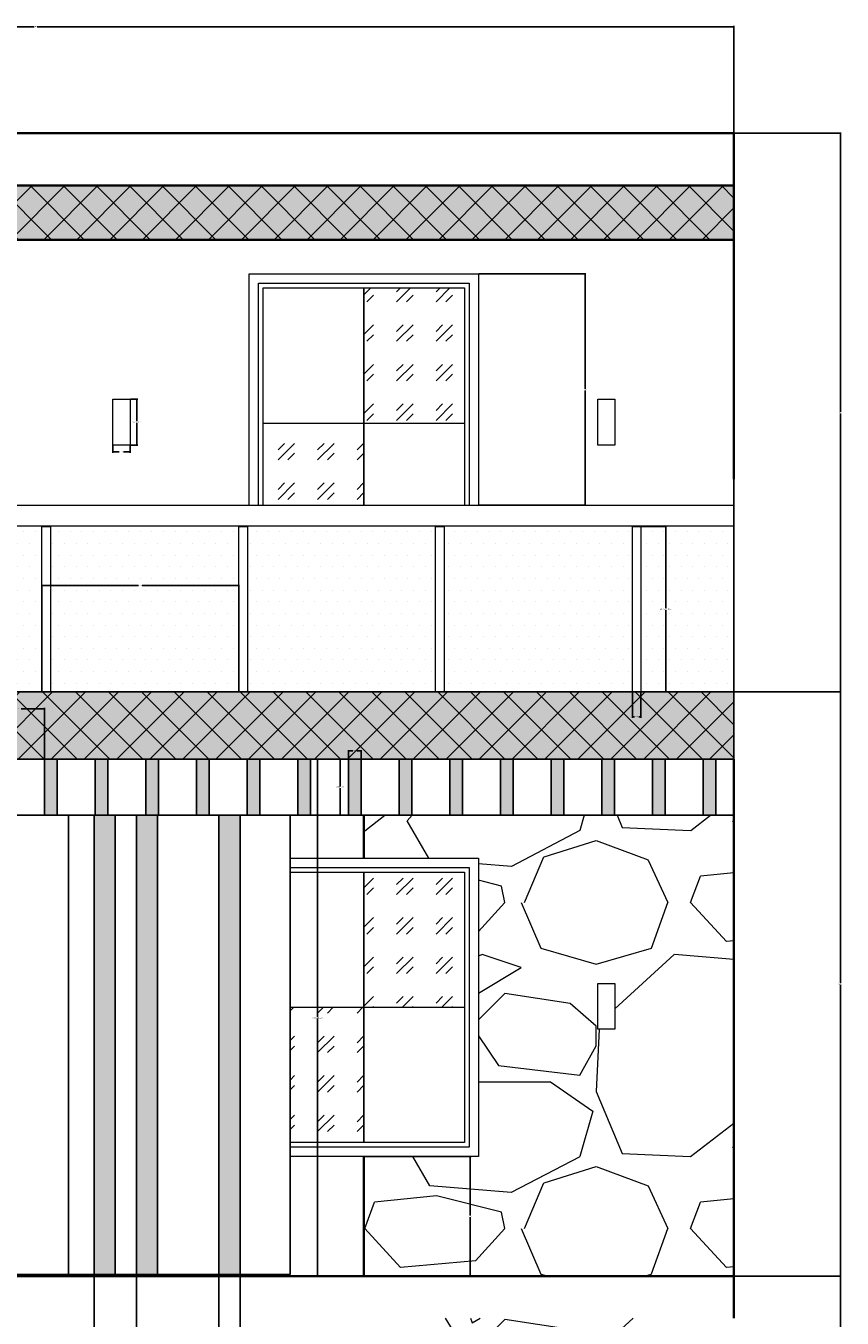
# Model space of a CAD drawing. Units: inches. Extents: x -13 to 333, y -76 to 399.
# Tile 3 of 3: x 158 to 333, y 121 to 399. Entities that reach past the tile are written whole.
import ezdxf

# ---------------------------------------------------------------- set-up
doc = ezdxf.new("R2010")
doc.units = ezdxf.units.IN
doc.header["$MEASUREMENT"] = 0
for name, color, linetype, lineweight in [('A-ANNO-DIMS', 2, 'Continuous', 18), ('A-ELEV-TRIM', 7, 'Continuous', 25), ('A-FLOR', 7, 'Continuous', 35), ('A-FLOR-HRAL', 4, 'Continuous', 20), ('A-FLOR-HRAL-PATT', 8, 'Continuous', 13), ('A-GLAZ', 4, 'Continuous', 18), ('A-GLAZ-PATT', 8, 'Continuous', 13), ('A-ROOF', 7, 'Continuous', 35), ('A-WALL', 7, 'Continuous', 35), ('A-WALL-PATT', 252, 'Continuous', 13), ('E-LITE-EXTR', 2, 'Continuous', 18)]:
    doc.layers.add(name, color=color, linetype=linetype, lineweight=lineweight)
doc.styles.get("Standard").update_dxf_attribs({"font": 'arial.ttf'})
doc.dimstyles.get("Standard").update_dxf_attribs({"dimtxt": 0.18, "dimasz": 0.18, "dimexe": 0.18, "dimexo": 0.0625, "dimgap": 0.09, "dimtad": 0, "dimtih": 1, "dimtoh": 1, "dimdec": 4, "dimzin": 0, "dimdsep": 46, "dimtxsty": 'Standard', "dimcen": 0.09, "dimadec": 0, "dimazin": 0, "dimtfac": 1, "dimtdec": 4, "dimtofl": 0, "dimtmove": 0, "dimatfit": 3, "dimfxl": 1, "dimtolj": 1, "dimtzin": 0, "dimarcsym": 0})

# ---------------------------------------------------------------- blocks, each defined once
blk = doc.blocks.new('LIGHT-WALL-SCONCE')
blk.add_lwpolyline([(0, 9.86), (3.7, 9.86), (3.7, 0), (0, 0)], close=True)
blk = doc.blocks.new('FASCIA-BATTEN')
blk.add_lwpolyline([(0, 12), (0, 0), (2.72, 0), (2.72, 12)])
blk = doc.blocks.new('GUARD-POST-TERRACE')
blk.add_lwpolyline([(0, 35.57), (1.84, 35.57), (1.84, 0), (0, 0)], close=True)
blk = doc.blocks.new('FACADE-VERTICAL-STRIP')
for points in [[(4.54, 111), (0, 111)], [(0, 99), (0, 0), (4.54, 0), (4.54, 99)]]:
    blk.add_lwpolyline(points)
blk = doc.blocks.new('*D6')
at = {"layer": 'A-ANNO-DIMS', "color": 0, "lineweight": -2, "transparency": 16777216}
for p, q in [((227.2, 241.18), (225.28, 241.18)), ((225.46, 241), (225.46, 235.36)), ((225.46, 229.36), (225.46, 235)), ((227.2, 229.18), (225.28, 229.18))]:
    blk.add_line(p, q, dxfattribs=at)
at = {"layer": 'A-ANNO-DIMS', "color": 0, "transparency": 16777216}
for points in [[(225.43, 241), (225.49, 241), (225.46, 241.18)], [(225.43, 229.36), (225.49, 229.36), (225.46, 229.18)]]:
    blk.add_solid(points, dxfattribs=at)
at = {"layer": 'Defpoints', "color": 0, "transparency": 16777216}
for p in [(225.46, 241.18), (227.26, 241.18), (227.26, 229.18)]:
    blk.add_point(p, dxfattribs=at)
at = {"layer": 'A-ANNO-DIMS', "color": 0, "transparency": 16777216, "insert": (225.46, 235.18), "char_height": 0.18, "attachment_point": 5}
blk.add_mtext('\\A1;BATTEN 12 TYP.', dxfattribs=at)
blk = doc.blocks.new('*D7')
at = {"layer": 'A-ANNO-DIMS', "color": 0, "lineweight": -2, "transparency": 16777216}
for p, q in [((227.26, 241.24), (227.26, 243.16)), ((227.44, 242.98), (228.17, 242.98)), ((229.8, 242.98), (229.08, 242.98)), ((229.98, 241.24), (229.98, 243.16))]:
    blk.add_line(p, q, dxfattribs=at)
at = {"layer": 'A-ANNO-DIMS', "color": 0, "transparency": 16777216}
for points in [[(227.44, 243.01), (227.44, 242.95), (227.26, 242.98)], [(229.8, 243.01), (229.8, 242.95), (229.98, 242.98)]]:
    blk.add_solid(points, dxfattribs=at)
at = {"layer": 'Defpoints', "color": 0, "transparency": 16777216}
for p in [(229.98, 242.98), (227.26, 241.18), (229.98, 241.18)]:
    blk.add_point(p, dxfattribs=at)
at = {"layer": 'A-ANNO-DIMS', "color": 0, "transparency": 16777216, "insert": (228.62, 242.98), "char_height": 0.18, "attachment_point": 5}
blk.add_mtext('\\A1;3 TYP.', dxfattribs=at)
blk = doc.blocks.new('*D8')
at = {"layer": 'A-ANNO-DIMS', "color": 0, "lineweight": -2, "transparency": 16777216}
for p, q in [((180.41, 318.52), (182.01, 318.52)), ((181.83, 318.34), (181.83, 313.77)), ((181.83, 308.83), (181.83, 313.4)), ((180.41, 308.65), (182.01, 308.65))]:
    blk.add_line(p, q, dxfattribs=at)
at = {"layer": 'A-ANNO-DIMS', "color": 0, "transparency": 16777216}
for points in [[(181.8, 318.34), (181.86, 318.34), (181.83, 318.52)], [(181.8, 308.83), (181.86, 308.83), (181.83, 308.65)]]:
    blk.add_solid(points, dxfattribs=at)
at = {"layer": 'Defpoints', "color": 0, "transparency": 16777216}
for p in [(180.35, 318.52), (181.83, 318.52), (180.35, 308.65)]:
    blk.add_point(p, dxfattribs=at)
at = {"layer": 'A-ANNO-DIMS', "color": 0, "transparency": 16777216, "insert": (181.83, 313.59), "char_height": 0.18, "attachment_point": 5}
blk.add_mtext('\\A1;SCONCE 10 TYP.', dxfattribs=at)
blk = doc.blocks.new('*D9')
at = {"layer": 'A-ANNO-DIMS', "color": 0, "lineweight": -2, "transparency": 16777216}
for p, q in [((176.65, 308.59), (176.65, 307)), ((180.35, 308.59), (180.35, 307)), ((176.83, 307.18), (178.04, 307.18)), ((180.17, 307.18), (178.96, 307.18))]:
    blk.add_line(p, q, dxfattribs=at)
at = {"layer": 'A-ANNO-DIMS', "color": 0, "transparency": 16777216}
for points in [[(176.83, 307.21), (176.83, 307.15), (176.65, 307.18)], [(180.17, 307.21), (180.17, 307.15), (180.35, 307.18)]]:
    blk.add_solid(points, dxfattribs=at)
at = {"layer": 'Defpoints', "color": 0, "transparency": 16777216}
for p in [(176.65, 308.65), (180.35, 308.65), (180.35, 307.18)]:
    blk.add_point(p, dxfattribs=at)
at = {"layer": 'A-ANNO-DIMS', "color": 0, "transparency": 16777216, "insert": (178.5, 307.18), "char_height": 0.18, "attachment_point": 5}
blk.add_mtext('\\A1;4 TYP.', dxfattribs=at)
blk = doc.blocks.new('*D10')
at = {"layer": 'A-ANNO-DIMS', "color": 0, "lineweight": -2, "transparency": 16777216}
for p, q in [((290.15, 291.2), (295.6, 291.2)), ((295.42, 291.02), (295.42, 273.6)), ((295.42, 255.81), (295.42, 273.23)), ((290.15, 255.63), (295.6, 255.63))]:
    blk.add_line(p, q, dxfattribs=at)
at = {"layer": 'A-ANNO-DIMS', "color": 0, "transparency": 16777216}
for points in [[(295.39, 291.02), (295.45, 291.02), (295.42, 291.2)], [(295.39, 255.81), (295.45, 255.81), (295.42, 255.63)]]:
    blk.add_solid(points, dxfattribs=at)
at = {"layer": 'Defpoints', "color": 0, "transparency": 16777216}
for p in [(290.08, 291.2), (295.42, 291.2), (290.08, 255.63)]:
    blk.add_point(p, dxfattribs=at)
at = {"layer": 'A-ANNO-DIMS', "color": 0, "transparency": 16777216, "insert": (295.42, 273.42), "char_height": 0.18, "attachment_point": 5}
blk.add_mtext('\\A1;TERRACE POST 36 TYP.', dxfattribs=at)
blk = doc.blocks.new('*D11')
at = {"layer": 'A-ANNO-DIMS', "color": 0, "lineweight": -2, "transparency": 16777216}
for p, q in [((288.25, 255.57), (288.25, 250.11)), ((290.08, 255.57), (290.08, 250.11)), ((288.43, 250.29), (288.71, 250.29)), ((289.9, 250.29), (289.63, 250.29))]:
    blk.add_line(p, q, dxfattribs=at)
at = {"layer": 'A-ANNO-DIMS', "color": 0, "transparency": 16777216}
for points in [[(288.43, 250.32), (288.43, 250.26), (288.25, 250.29)], [(289.9, 250.32), (289.9, 250.26), (290.08, 250.29)]]:
    blk.add_solid(points, dxfattribs=at)
at = {"layer": 'Defpoints', "color": 0, "transparency": 16777216}
for p in [(288.25, 255.63), (290.08, 255.63), (290.08, 250.29)]:
    blk.add_point(p, dxfattribs=at)
at = {"layer": 'A-ANNO-DIMS', "color": 0, "transparency": 16777216, "insert": (289.17, 250.29), "char_height": 0.18, "attachment_point": 5}
blk.add_mtext('\\A1;2 TYP.', dxfattribs=at)
blk = doc.blocks.new('*D14')
at = {"layer": 'A-ANNO-DIMS', "color": 0, "lineweight": -2, "transparency": 16777216}
for p, q in [((204.05, 241.18), (220.82, 241.18)), ((220.64, 241), (220.64, 185.86)), ((220.64, 130.36), (220.64, 185.49)), ((204.05, 130.18), (220.82, 130.18))]:
    blk.add_line(p, q, dxfattribs=at)
at = {"layer": 'A-ANNO-DIMS', "color": 0, "transparency": 16777216}
for points in [[(220.61, 241), (220.67, 241), (220.64, 241.18)], [(220.61, 130.36), (220.67, 130.36), (220.64, 130.18)]]:
    blk.add_solid(points, dxfattribs=at)
at = {"layer": 'Defpoints', "color": 0, "transparency": 16777216}
for p in [(203.99, 241.18), (220.64, 241.18), (203.99, 130.18)]:
    blk.add_point(p, dxfattribs=at)
at = {"layer": 'A-ANNO-DIMS', "color": 0, "transparency": 16777216, "insert": (220.64, 185.68), "char_height": 0.18, "attachment_point": 5}
blk.add_mtext('\\A1;FACADE STRIP 111 TYP.', dxfattribs=at)
blk = doc.blocks.new('*D15')
at = {"layer": 'A-ANNO-DIMS', "color": 0, "lineweight": -2, "transparency": 16777216}
for p, q in [((199.44, 130.11), (199.44, 113.35)), ((203.99, 130.11), (203.99, 113.35)), ((199.62, 113.53), (201.26, 113.53)), ((203.81, 113.53), (202.17, 113.53))]:
    blk.add_line(p, q, dxfattribs=at)
at = {"layer": 'A-ANNO-DIMS', "color": 0, "transparency": 16777216}
for points in [[(199.62, 113.56), (199.62, 113.5), (199.44, 113.53)], [(203.81, 113.56), (203.81, 113.5), (203.99, 113.53)]]:
    blk.add_solid(points, dxfattribs=at)
at = {"layer": 'Defpoints', "color": 0, "transparency": 16777216}
for p in [(199.44, 130.18), (203.99, 130.18), (203.99, 113.53)]:
    blk.add_point(p, dxfattribs=at)
at = {"layer": 'A-ANNO-DIMS', "color": 0, "transparency": 16777216, "insert": (201.71, 113.53), "char_height": 0.18, "attachment_point": 5}
blk.add_mtext('\\A1;5 TYP.', dxfattribs=at)
blk = doc.blocks.new('*D16')
at = {"layer": 'A-ANNO-DIMS', "color": 0, "lineweight": -2, "transparency": 16777216}
for p, q in [((10.07, 301.43), (10.07, 398.67)), ((10.25, 398.49), (159.78, 398.49)), ((309.89, 398.49), (160.36, 398.49)), ((310.07, 375.69), (310.07, 398.67))]:
    blk.add_line(p, q, dxfattribs=at)
at = {"layer": 'A-ANNO-DIMS', "color": 0, "transparency": 16777216}
for points in [[(10.25, 398.52), (10.25, 398.46), (10.07, 398.49)], [(309.89, 398.52), (309.89, 398.46), (310.07, 398.49)]]:
    blk.add_solid(points, dxfattribs=at)
at = {"layer": 'Defpoints', "color": 0, "transparency": 16777216}
for p in [(310.07, 398.49), (310.07, 375.63), (10.07, 301.36)]:
    blk.add_point(p, dxfattribs=at)
at = {"layer": 'A-ANNO-DIMS', "color": 0, "transparency": 16777216, "insert": (160.07, 398.49), "char_height": 0.18, "attachment_point": 5}
blk.add_mtext('\\A1;300', dxfattribs=at)
blk = doc.blocks.new('*D19')
at = {"layer": 'A-ANNO-DIMS', "color": 0, "lineweight": -2, "transparency": 16777216}
for p, q in [((310.13, 130.18), (333.11, 130.18)), ((332.93, 130), (332.93, 65.86)), ((332.93, 1.36), (332.93, 65.49)), ((310.13, 1.18), (333.11, 1.18))]:
    blk.add_line(p, q, dxfattribs=at)
at = {"layer": 'A-ANNO-DIMS', "color": 0, "transparency": 16777216}
for points in [[(332.9, 130), (332.96, 130), (332.93, 130.18)], [(332.9, 1.36), (332.96, 1.36), (332.93, 1.18)]]:
    blk.add_solid(points, dxfattribs=at)
at = {"layer": 'Defpoints', "color": 0, "transparency": 16777216}
for p in [(310.07, 130.18), (332.93, 130.18), (310.07, 1.18)]:
    blk.add_point(p, dxfattribs=at)
at = {"layer": 'A-ANNO-DIMS', "color": 0, "transparency": 16777216, "insert": (332.93, 65.68), "char_height": 0.18, "attachment_point": 5}
blk.add_mtext('\\A1;129', dxfattribs=at)
blk = doc.blocks.new('*D20')
at = {"layer": 'A-ANNO-DIMS', "color": 0, "lineweight": -2, "transparency": 16777216}
for p, q in [((310.13, 255.63), (333.11, 255.63)), ((332.93, 255.45), (332.93, 193.09)), ((332.93, 130.36), (332.93, 192.72)), ((310.13, 130.18), (333.11, 130.18))]:
    blk.add_line(p, q, dxfattribs=at)
at = {"layer": 'A-ANNO-DIMS', "color": 0, "transparency": 16777216}
for points in [[(332.9, 255.45), (332.96, 255.45), (332.93, 255.63)], [(332.9, 130.36), (332.96, 130.36), (332.93, 130.18)]]:
    blk.add_solid(points, dxfattribs=at)
at = {"layer": 'Defpoints', "color": 0, "transparency": 16777216}
for p in [(310.07, 255.63), (332.93, 255.63), (310.07, 130.18)]:
    blk.add_point(p, dxfattribs=at)
at = {"layer": 'A-ANNO-DIMS', "color": 0, "transparency": 16777216, "insert": (332.93, 192.9), "char_height": 0.18, "attachment_point": 5}
blk.add_mtext('\\A1;125.46', dxfattribs=at)
blk = doc.blocks.new('*D21')
at = {"layer": 'A-ANNO-DIMS', "color": 0, "lineweight": -2, "transparency": 16777216}
for p, q in [((310.13, 375.63), (333.11, 375.63)), ((332.93, 375.45), (332.93, 315.81)), ((332.93, 255.81), (332.93, 315.45)), ((310.13, 255.63), (333.11, 255.63))]:
    blk.add_line(p, q, dxfattribs=at)
at = {"layer": 'A-ANNO-DIMS', "color": 0, "transparency": 16777216}
for points in [[(332.9, 375.45), (332.96, 375.45), (332.93, 375.63)], [(332.9, 255.81), (332.96, 255.81), (332.93, 255.63)]]:
    blk.add_solid(points, dxfattribs=at)
at = {"layer": 'Defpoints', "color": 0, "transparency": 16777216}
for p in [(310.07, 375.63), (332.93, 375.63), (310.07, 255.63)]:
    blk.add_point(p, dxfattribs=at)
at = {"layer": 'A-ANNO-DIMS', "color": 0, "transparency": 16777216, "insert": (332.93, 315.63), "char_height": 0.18, "attachment_point": 5}
blk.add_mtext('\\A1;120', dxfattribs=at)
blk = doc.blocks.new('*D35')
at = {"layer": 'A-ANNO-DIMS', "color": 0, "lineweight": -2, "transparency": 16777216}
for p, q in [((161.43, 255.69), (161.43, 278.67)), ((161.61, 278.49), (182.17, 278.49)), ((203.52, 278.49), (182.96, 278.49)), ((203.7, 255.69), (203.7, 278.67))]:
    blk.add_line(p, q, dxfattribs=at)
at = {"layer": 'A-ANNO-DIMS', "color": 0, "transparency": 16777216}
for points in [[(161.61, 278.52), (161.61, 278.46), (161.43, 278.49)], [(203.52, 278.52), (203.52, 278.46), (203.7, 278.49)]]:
    blk.add_solid(points, dxfattribs=at)
at = {"layer": 'Defpoints', "color": 0, "transparency": 16777216}
for p in [(203.7, 278.49), (161.43, 255.63), (203.7, 255.63)]:
    blk.add_point(p, dxfattribs=at)
at = {"layer": 'A-ANNO-DIMS', "color": 0, "transparency": 16777216, "insert": (182.56, 278.49), "char_height": 0.18, "attachment_point": 5}
blk.add_mtext('\\A1;42.27', dxfattribs=at)
blk = doc.blocks.new('*D36')
at = {"layer": 'A-ANNO-DIMS', "color": 0, "lineweight": -2, "transparency": 16777216}
for p, q in [((151.07, 229.24), (151.07, 252.22)), ((151.25, 252.04), (156.06, 252.04)), ((161.78, 252.04), (156.97, 252.04)), ((161.96, 229.24), (161.96, 252.22))]:
    blk.add_line(p, q, dxfattribs=at)
at = {"layer": 'A-ANNO-DIMS', "color": 0, "transparency": 16777216}
for points in [[(151.25, 252.07), (151.25, 252.01), (151.07, 252.04)], [(161.78, 252.07), (161.78, 252.01), (161.96, 252.04)]]:
    blk.add_solid(points, dxfattribs=at)
at = {"layer": 'Defpoints', "color": 0, "transparency": 16777216}
for p in [(161.96, 252.04), (151.07, 229.18), (161.96, 229.18)]:
    blk.add_point(p, dxfattribs=at)
at = {"layer": 'A-ANNO-DIMS', "color": 0, "transparency": 16777216, "insert": (156.51, 252.04), "char_height": 0.18, "attachment_point": 5}
blk.add_mtext('\\A1;10.885', dxfattribs=at)
blk = doc.blocks.new('*D41')
at = {"layer": 'A-ANNO-DIMS', "color": 0, "lineweight": -2, "transparency": 16777216}
for p, q in [((255.28, 345.41), (278.25, 345.41)), ((278.07, 345.23), (278.07, 320.75)), ((278.07, 295.9), (278.07, 320.38)), ((255.28, 295.72), (278.25, 295.72))]:
    blk.add_line(p, q, dxfattribs=at)
at = {"layer": 'A-ANNO-DIMS', "color": 0, "transparency": 16777216}
for points in [[(278.04, 345.23), (278.1, 345.23), (278.07, 345.41)], [(278.04, 295.9), (278.1, 295.9), (278.07, 295.72)]]:
    blk.add_solid(points, dxfattribs=at)
at = {"layer": 'Defpoints', "color": 0, "transparency": 16777216}
for p in [(255.21, 345.41), (255.21, 295.72), (278.07, 295.72)]:
    blk.add_point(p, dxfattribs=at)
at = {"layer": 'A-ANNO-DIMS', "color": 0, "transparency": 16777216, "insert": (278.07, 320.57), "char_height": 0.18, "attachment_point": 5}
blk.add_mtext('\\A1;49.68', dxfattribs=at)
blk = doc.blocks.new('*D43')
at = {"layer": 'A-ANNO-DIMS', "color": 0, "lineweight": -2, "transparency": 16777216}
for p, q in [((151.07, 130.11), (151.07, 107.14)), ((172.62, 130.11), (172.62, 107.14)), ((151.25, 107.32), (161.38, 107.32)), ((172.44, 107.32), (162.31, 107.32))]:
    blk.add_line(p, q, dxfattribs=at)
at = {"layer": 'A-ANNO-DIMS', "color": 0, "transparency": 16777216}
for points in [[(151.25, 107.35), (151.25, 107.29), (151.07, 107.32)], [(172.44, 107.35), (172.44, 107.29), (172.62, 107.32)]]:
    blk.add_solid(points, dxfattribs=at)
at = {"layer": 'Defpoints', "color": 0, "transparency": 16777216}
for p in [(151.07, 130.18), (172.62, 130.18), (151.07, 107.32)]:
    blk.add_point(p, dxfattribs=at)
at = {"layer": 'A-ANNO-DIMS', "color": 0, "transparency": 16777216, "insert": (161.84, 107.32), "char_height": 0.18, "attachment_point": 5}
blk.add_mtext('\\A1;21.545', dxfattribs=at)
blk = doc.blocks.new('*D44')
at = {"layer": 'A-ANNO-DIMS', "color": 0, "lineweight": -2, "transparency": 16777216}
for p, q in [((172.62, 130.11), (172.62, 107.14)), ((181.7, 130.11), (181.7, 107.14)), ((172.8, 107.32), (176.83, 107.32)), ((181.52, 107.32), (177.48, 107.32))]:
    blk.add_line(p, q, dxfattribs=at)
at = {"layer": 'A-ANNO-DIMS', "color": 0, "transparency": 16777216}
for points in [[(172.8, 107.35), (172.8, 107.29), (172.62, 107.32)], [(181.52, 107.35), (181.52, 107.29), (181.7, 107.32)]]:
    blk.add_solid(points, dxfattribs=at)
at = {"layer": 'Defpoints', "color": 0, "transparency": 16777216}
for p in [(172.62, 130.18), (181.7, 130.18), (172.62, 107.32)]:
    blk.add_point(p, dxfattribs=at)
at = {"layer": 'A-ANNO-DIMS', "color": 0, "transparency": 16777216, "insert": (177.16, 107.32), "char_height": 0.18, "attachment_point": 5}
blk.add_mtext('\\A1;9.08', dxfattribs=at)
blk = doc.blocks.new('*D45')
at = {"layer": 'A-ANNO-DIMS', "color": 0, "lineweight": -2, "transparency": 16777216}
for p, q in [((181.7, 130.11), (181.7, 107.14)), ((199.44, 130.11), (199.44, 107.14)), ((181.88, 107.32), (190.18, 107.32)), ((199.26, 107.32), (190.96, 107.32))]:
    blk.add_line(p, q, dxfattribs=at)
at = {"layer": 'A-ANNO-DIMS', "color": 0, "transparency": 16777216}
for points in [[(181.88, 107.35), (181.88, 107.29), (181.7, 107.32)], [(199.26, 107.35), (199.26, 107.29), (199.44, 107.32)]]:
    blk.add_solid(points, dxfattribs=at)
at = {"layer": 'Defpoints', "color": 0, "transparency": 16777216}
for p in [(181.7, 130.18), (199.44, 130.18), (181.7, 107.32)]:
    blk.add_point(p, dxfattribs=at)
at = {"layer": 'A-ANNO-DIMS', "color": 0, "transparency": 16777216, "insert": (190.57, 107.32), "char_height": 0.18, "attachment_point": 5}
blk.add_mtext('\\A1;17.75', dxfattribs=at)
blk = doc.blocks.new('*D48')
at = {"layer": 'A-ANNO-DIMS', "color": 0, "lineweight": -2, "transparency": 16777216}
for p, q in [((230.63, 155.9), (253.61, 155.9)), ((253.43, 155.72), (253.43, 143.22)), ((253.43, 130.36), (253.43, 142.86)), ((230.63, 130.18), (253.61, 130.18))]:
    blk.add_line(p, q, dxfattribs=at)
at = {"layer": 'A-ANNO-DIMS', "color": 0, "transparency": 16777216}
for points in [[(253.4, 155.72), (253.46, 155.72), (253.43, 155.9)], [(253.4, 130.36), (253.46, 130.36), (253.43, 130.18)]]:
    blk.add_solid(points, dxfattribs=at)
at = {"layer": 'Defpoints', "color": 0, "transparency": 16777216}
for p in [(230.57, 155.9), (230.57, 130.18), (253.43, 130.18)]:
    blk.add_point(p, dxfattribs=at)
at = {"layer": 'A-ANNO-DIMS', "color": 0, "transparency": 16777216, "insert": (253.43, 143.04), "char_height": 0.18, "attachment_point": 5}
blk.add_mtext('\\A1;25.723', dxfattribs=at)

msp = doc.modelspace()

# ---------------------------------------------------------------- hatches: boundary and pattern name
at = {"layer": 'A-FLOR-HRAL-PATT'}
h = msp.add_hatch(dxfattribs=at)
h.set_pattern_fill('DOTS', color=256, scale=40, style=0)
h.paths.add_polyline_path([(120.9893, 255.6309), (161.426, 255.6309), (161.426, 291.2047), (120.9893, 291.2047)])
h.paths.add_polyline_path([(163.2631, 255.6309), (203.6999, 255.6309), (203.6999, 291.2047), (163.2631, 291.2047)], flags=0)
h.paths.add_polyline_path([(205.537, 255.6309), (245.9737, 255.6309), (245.9737, 291.2047), (205.537, 291.2047)], flags=0)
h.paths.add_polyline_path([(247.8108, 255.6309), (288.2475, 255.6309), (288.2475, 291.2047), (247.8108, 291.2047)], flags=0)
h.paths.add_polyline_path([(290.0846, 255.6309), (310.0707, 255.6309), (310.0707, 291.2047), (290.0846, 291.2047)], flags=0)
at = {"layer": 'A-GLAZ-PATT', "transparency": 33554595}
h = msp.add_hatch(dxfattribs=at)
h.set_pattern_fill('GOST_GLASS', color=256)
h.set_pattern_definition([(45, (0, 0), (8.48528, 0), [5, -7]), (45, (2.1213, 0), (8.48528, 0), [2, -10]), (45, (0, 2.1213), (8.48528, 0), [2, -10])])
h.paths.add_polyline_path([(252.2145, 216.9526), (230.5707, 216.9526), (230.5707, 187.9258), (252.2145, 187.9258)])
h.paths.add_polyline_path([(230.5707, 187.9258), (214.7169, 187.9258), (214.7169, 158.899), (230.5707, 158.899)])
h.paths.add_polyline_path([(252.2145, 87.9526), (230.5707, 87.9526), (230.5707, 58.9258), (252.2145, 58.9258)])
h.paths.add_polyline_path([(230.5707, 58.9258), (208.9269, 58.9258), (208.9269, 29.899), (230.5707, 29.899)])
h.paths.add_polyline_path([(252.2145, 342.4077), (230.5707, 342.4077), (230.5707, 313.3809), (252.2145, 313.3809)])
h.paths.add_polyline_path([(230.5707, 313.3809), (208.9269, 313.3809), (208.9269, 295.7236), (230.5707, 295.7236)])
at = {"layer": 'A-WALL-PATT', "transparency": 33554556}
h = msp.add_hatch(dxfattribs=at)
h.set_pattern_fill('ANSI37', color=256, scale=40)
h.paths.add_polyline_path([(51.3479, 271.2697), (10.0707, 271.2697), (10.0707, 241.1758), (10.0707, 228.0051), (24.6528, 228.0051, -0.28286751), (46.0707, 241.1758), (310.0707, 241.1758), (310.0707, 255.6309), (67.3439, 255.6309, 0.40761741)])
h.paths.add_polyline_path([(80.2381, 352.7454), (310.0707, 352.7454), (310.0707, 364.3576), (80.2381, 364.3576), (68.6976, 364.3576), (68.6976, 301.3637), (80.2381, 301.3637)])
at = {"layer": 'A-WALL-PATT', "transparency": 33554595}
h = msp.add_hatch(color=256, dxfattribs=at)
h.dxf.hatch_style = 1
h.set_gradient(color1=(175, 217, 170), color2=(175, 217, 170))
h.paths.add_polyline_path([(310.0707, 364.3576), (80.2381, 364.3576), (68.6976, 364.3576), (68.6976, 301.3637), (80.2381, 301.3637), (80.2381, 352.7454), (310.0707, 352.7454)])
h.paths.add_polyline_path([(51.3479, 271.2697), (10.0707, 271.2697), (10.0707, 241.1758), (10.0707, 228.0051), (24.6528, 228.0051, -0.28286751), (46.0707, 241.1758), (310.0707, 241.1758), (310.0707, 255.6309), (67.3439, 255.6309, 0.40761741)])
at = {"layer": 'A-WALL-PATT', "transparency": 33554531}
h = msp.add_hatch(color=256, dxfattribs=at)
h.dxf.hatch_style = 1
h.set_gradient(color1=(205, 105, 40), color2=(205, 105, 40), name='INVCURVED')
h.paths.add_polyline_path([(153.7927, 241.1758), (151.0707, 241.1758), (151.0707, 229.1758), (153.7927, 229.1758)])
h.paths.add_polyline_path([(164.6773, 241.1758), (161.9553, 241.1758), (161.9553, 229.1758), (164.6773, 229.1758)])
h.paths.add_polyline_path([(175.5619, 241.1758), (172.8398, 241.1758), (172.8398, 229.1758), (175.5619, 229.1758)])
h.paths.add_polyline_path([(186.4464, 241.1758), (183.7244, 241.1758), (183.7244, 229.1758), (186.4464, 229.1758)])
h.paths.add_polyline_path([(197.331, 241.1758), (194.609, 241.1758), (194.609, 229.1758), (197.331, 229.1758)])
h.paths.add_polyline_path([(208.2156, 241.1758), (205.4936, 241.1758), (205.4936, 229.1758), (208.2156, 229.1758)])
h.paths.add_polyline_path([(219.1001, 241.1758), (216.3781, 241.1758), (216.3781, 229.1758), (219.1001, 229.1758)])
h.paths.add_polyline_path([(229.9847, 241.1758), (227.2627, 241.1758), (227.2627, 229.1758), (229.9847, 229.1758)])
h.paths.add_polyline_path([(240.8693, 241.1758), (238.1473, 241.1758), (238.1473, 229.1758), (240.8693, 229.1758)])
h.paths.add_polyline_path([(251.7539, 241.1758), (249.0319, 241.1758), (249.0319, 229.1758), (251.7539, 229.1758)])
h.paths.add_polyline_path([(262.6384, 241.1758), (259.9164, 241.1758), (259.9164, 229.1758), (262.6384, 229.1758)])
h.paths.add_polyline_path([(273.523, 241.1758), (270.801, 241.1758), (270.801, 229.1758), (273.523, 229.1758)])
h.paths.add_polyline_path([(284.4076, 241.1758), (281.6856, 241.1758), (281.6856, 229.1758), (284.4076, 229.1758)])
h.paths.add_polyline_path([(295.2921, 241.1758), (292.5701, 241.1758), (292.5701, 229.1758), (295.2921, 229.1758)])
h.paths.add_polyline_path([(306.1767, 241.1758), (303.4547, 241.1758), (303.4547, 229.1758), (306.1767, 229.1758)])
at = {"layer": 'A-WALL-PATT', "transparency": 33554595}
h = msp.add_hatch(color=256, dxfattribs=at)
h.dxf.hatch_style = 1
h.set_gradient(color1=(94, 103, 175), color2=(169, 83, 160), name='CURVED')
h.paths.add_polyline_path([(177.1558, 229.1758), (172.6155, 229.1758), (172.6155, 130.5549), (177.1558, 130.5549)])
h.paths.add_polyline_path([(186.2365, 229.1758), (183.7244, 229.1758), (181.6962, 229.1758), (181.6962, 130.5549), (186.2365, 130.5549)])
h.paths.add_polyline_path([(203.9852, 229.1758), (199.4448, 229.1758), (199.4448, 130.5549), (203.9852, 130.5549)])
h = msp.add_hatch(dxfattribs=at)
h.set_pattern_fill('GRAVEL', color=256, scale=70)
h.paths.add_polyline_path([(310.0707, 121.1758), (230.5707, 121.1758), (230.5707, 90.9526), (255.2145, 90.9526), (255.2145, 26.899), (230.5707, 26.899), (230.5707, 1.1758), (310.0707, 1.1758)])
h.paths.add_polyline_path([(280.7936, 64.0624), (284.4916, 64.0624), (284.4916, 54.1998), (280.7936, 54.1998)], flags=16)
h.paths.add_polyline_path([(310.0707, 229.1758), (230.5707, 229.1758), (230.5707, 219.9526), (255.2145, 219.9526), (255.2145, 155.899), (230.5707, 155.899), (230.5707, 130.1758), (310.0707, 130.1758)])
h.paths.add_polyline_path([(280.7936, 183.1998), (280.7936, 193.0624), (284.4916, 193.0624), (284.4916, 183.1998)], flags=16)

# ---------------------------------------------------------------- linework, layer by layer
at = {"layer": 'A-ELEV-TRIM'}
for p, q in [((67.3439, 255.6309), (310.0707, 255.6309)), ((46.0707, 241.1758), (310.0707, 241.1758)), ((58.0707, 229.1758), (310.0707, 229.1758))]:
    msp.add_line(p, q, dxfattribs=at)
for points in [[(46.0707, 241.1758), (310.0707, 241.1758), (310.0707, 301.3637)], [(151.0707, 241.1758), (167.1016, 241.1758)], [(214.7169, 241.1758), (167.1016, 241.1758)], [(167.1016, 229.1758), (167.1016, 130.5549), (151.0707, 130.5549), (151.0707, 229.1758)], [(167.1016, 229.1758), (167.1016, 130.5549), (214.7169, 130.5549), (214.7169, 229.1758)]]:
    msp.add_lwpolyline(points, dxfattribs=at)
at = {"layer": 'A-FLOR'}
msp.add_line((310.0707, 130.1758), (10.0707, 130.1758), dxfattribs=at)
at = {"layer": 'A-FLOR-HRAL'}
msp.add_lwpolyline([(120.9893, 295.7236), (310.0707, 295.7236), (310.0707, 291.2047), (120.9893, 291.2047)], close=True, dxfattribs=at)
at = {"layer": 'A-GLAZ'}
for p, q in [((230.5707, 342.4077), (230.5707, 295.7236)), ((230.5707, 295.7236), (230.5707, 342.4077)), ((208.9269, 313.3809), (252.2145, 313.3809)), ((230.5707, 216.9526), (230.5707, 158.899)), ((230.5707, 158.899), (230.5707, 216.9526)), ((214.7169, 187.9258), (252.2145, 187.9258))]:
    msp.add_line(p, q, dxfattribs=at)
for points in [[(205.9269, 295.7236), (205.9269, 345.4077), (255.2145, 345.4077), (255.2145, 295.7236)], [(207.9269, 295.7236), (207.9269, 343.4077), (253.2145, 343.4077), (253.2145, 295.7236)], [(208.9269, 295.7236), (208.9269, 342.4077), (252.2145, 342.4077), (252.2145, 295.7236)], [(214.7169, 219.9526), (255.2145, 219.9526), (255.2145, 155.899), (214.7169, 155.899)], [(214.7169, 217.9526), (253.2145, 217.9526), (253.2145, 157.899), (214.7169, 157.899)], [(214.7169, 216.9526), (252.2145, 216.9526), (252.2145, 158.899), (214.7169, 158.899)]]:
    msp.add_lwpolyline(points, dxfattribs=at)
at = {"layer": 'A-ROOF'}
for p, q in [((310.0707, 375.6309), (151.0707, 375.6309)), ((310.0707, 301.3637), (310.0707, 375.6309))]:
    msp.add_line(p, q, dxfattribs=at)
msp.add_lwpolyline([(80.2381, 352.7454), (310.0707, 352.7454), (310.0707, 364.3576), (80.2381, 364.3576)], dxfattribs=at)
at = {"layer": 'A-WALL'}
for p, q in [((310.0707, 241.1758), (310.0707, 121.1758)), ((230.5707, 219.9526), (230.5707, 229.1758)), ((230.5707, 130.1758), (230.5707, 155.899))]:
    msp.add_line(p, q, dxfattribs=at)

# ---------------------------------------------------------------- block references
at = {"layer": 'A-ELEV-TRIM'}
for name, p in [('FASCIA-BATTEN', (161.9553, 229.1758)), ('FACADE-VERTICAL-STRIP', (172.6155, 130.1758)), ('FASCIA-BATTEN', (172.8398, 229.1758)), ('FACADE-VERTICAL-STRIP', (181.6962, 130.1758)), ('FASCIA-BATTEN', (183.7244, 229.1758)), ('FASCIA-BATTEN', (194.609, 229.1758)), ('FACADE-VERTICAL-STRIP', (199.4448, 130.1758)), ('FASCIA-BATTEN', (205.4936, 229.1758)), ('FASCIA-BATTEN', (216.3781, 229.1758)), ('FASCIA-BATTEN', (227.2627, 229.1758)), ('FASCIA-BATTEN', (238.1473, 229.1758)), ('FASCIA-BATTEN', (249.0319, 229.1758)), ('FASCIA-BATTEN', (259.9164, 229.1758)), ('FASCIA-BATTEN', (270.801, 229.1758)), ('FASCIA-BATTEN', (281.6856, 229.1758)), ('FASCIA-BATTEN', (292.5701, 229.1758)), ('FASCIA-BATTEN', (303.4547, 229.1758))]:
    msp.add_blockref(name, p, dxfattribs=at)
at = {"layer": 'A-FLOR-HRAL'}
for p in [(161.426, 255.6309), (203.6999, 255.6309), (245.9737, 255.6309), (288.2475, 255.6309)]:
    msp.add_blockref('GUARD-POST-TERRACE', p, dxfattribs=at)
at = {"layer": 'E-LITE-EXTR'}
for p in [(176.6498, 308.6549), (280.7936, 308.6549), (280.7936, 183.1998)]:
    msp.add_blockref('LIGHT-WALL-SCONCE', p, dxfattribs=at)

# ---------------------------------------------------------------- dimensions: what is measured, and where the dimension line sits
at = {"layer": 'A-ANNO-DIMS'}
for base, p1, p2, override, picture, middle in [((310.0707, 398.4909), (10.0707, 301.3637), (310.0707, 375.6309), {"dimdec": 0, "dimlfac": 1, "dimrnd": 0, "dimzin": 0, "dimdsep": 46, "dimlunit": 2}, '*D16', (160.0707, 398.4909)), ((203.6999, 278.4909), (161.426, 255.6309), (203.6999, 255.6309), {"dimdec": 2, "dimlfac": 1, "dimrnd": 0, "dimzin": 0, "dimdsep": 46, "dimlunit": 2}, '*D35', (182.5629, 278.4909)), ((161.9553, 252.0358), (151.0707, 229.1758), (161.9553, 229.1758), {"dimdec": 3, "dimlfac": 1, "dimrnd": 0, "dimzin": 0, "dimdsep": 46, "dimlunit": 2}, '*D36', (156.513, 252.0358))]:
    dim = msp.add_linear_dim(base=base, p1=p1, p2=p2, dimstyle='Standard', override=override, dxfattribs=at)
    dim.commit()
    dim.dimension.update_dxf_attribs({"geometry": picture, "text_midpoint": middle})
for base, p1, p2, angle, override, picture, middle in [((332.9307, 375.6309), (310.0707, 255.6309), (310.0707, 375.6309), 90, {"dimdec": 0, "dimlfac": 1, "dimrnd": 0, "dimzin": 0, "dimdsep": 46, "dimlunit": 2}, '*D21', (332.9307, 315.6309)), ((278.0745, 295.7236), (255.2145, 345.4077), (255.2145, 295.7236), 270, {"dimdec": 2, "dimlfac": 1, "dimrnd": 0, "dimzin": 0, "dimdsep": 46, "dimlunit": 2}, '*D41', (278.0745, 320.5656)), ((332.9307, 255.6309), (310.0707, 130.1758), (310.0707, 255.6309), 90, {"dimdec": 2, "dimlfac": 1, "dimrnd": 0, "dimzin": 0, "dimdsep": 46, "dimlunit": 2}, '*D20', (332.9307, 192.9033)), ((253.4307, 130.1758), (230.5707, 155.899), (230.5707, 130.1758), 270, {"dimdec": 3, "dimlfac": 1, "dimrnd": 0, "dimzin": 0, "dimdsep": 46, "dimlunit": 2}, '*D48', (253.4307, 143.0374)), ((151.0707, 107.3158), (172.6155, 130.1758), (151.0707, 130.1758), 180, {"dimdec": 3, "dimlfac": 1, "dimrnd": 0, "dimzin": 0, "dimdsep": 46, "dimlunit": 2}, '*D43', (161.8431, 107.3158)), ((172.6155, 107.3158), (181.6962, 130.1758), (172.6155, 130.1758), 180, {"dimdec": 2, "dimlfac": 1, "dimrnd": 0, "dimzin": 0, "dimdsep": 46, "dimlunit": 2}, '*D44', (177.1558, 107.3158)), ((181.6962, 107.3158), (199.4448, 130.1758), (181.6962, 130.1758), 180, {"dimdec": 2, "dimlfac": 1, "dimrnd": 0, "dimzin": 0, "dimdsep": 46, "dimlunit": 2}, '*D45', (190.5705, 107.3158)), ((332.9307, 130.1758), (310.0707, 1.1758), (310.0707, 130.1758), 90, {"dimdec": 0, "dimlfac": 1, "dimrnd": 0, "dimzin": 0, "dimdsep": 46, "dimlunit": 2}, '*D19', (332.9307, 65.6758))]:
    dim = msp.add_linear_dim(base=base, p1=p1, p2=p2, angle=angle, dimstyle='Standard', override=override, dxfattribs=at)
    dim.commit()
    dim.dimension.update_dxf_attribs({"geometry": picture, "text_midpoint": middle})
for base, p1, p2, text, picture, middle in [((181.8272, 318.5175), (180.3478, 308.6549), (180.3478, 318.5175), 'SCONCE <> TYP.', '*D8', (181.8272, 313.5862)), ((295.4207, 291.2047), (290.0846, 255.6309), (290.0846, 291.2047), 'TERRACE POST <> TYP.', '*D10', (295.4207, 273.4178)), ((220.6352, 241.1758), (203.9852, 130.1758), (203.9852, 241.1758), 'FACADE STRIP <> TYP.', '*D14', (220.6352, 185.6758)), ((225.4627, 241.1758), (227.2627, 229.1758), (227.2627, 241.1758), 'BATTEN <> TYP.', '*D6', (225.4627, 235.1758))]:
    dim = msp.add_linear_dim(base=base, p1=p1, p2=p2, angle=90, text=text, dimstyle='Standard', override={"dimdec": 0, "dimlfac": 1, "dimrnd": 0, "dimzin": 0, "dimdsep": 46, "dimlunit": 2}, dxfattribs=at)
    dim.commit()
    dim.dimension.update_dxf_attribs({"geometry": picture, "text_midpoint": middle})
for base, p1, p2, picture, middle in [((180.3478, 307.1756), (176.6498, 308.6549), (180.3478, 308.6549), '*D9', (178.4988, 307.1756)), ((290.0846, 250.2948), (288.2475, 255.6309), (290.0846, 255.6309), '*D11', (289.1661, 250.2948)), ((229.9847, 242.9758), (227.2627, 241.1758), (229.9847, 241.1758), '*D7', (228.6237, 242.9758)), ((203.9852, 113.5258), (199.4448, 130.1758), (203.9852, 130.1758), '*D15', (201.715, 113.5258))]:
    dim = msp.add_linear_dim(base=base, p1=p1, p2=p2, text='<> TYP.', dimstyle='Standard', override={"dimdec": 0, "dimlfac": 1, "dimrnd": 0, "dimzin": 0, "dimdsep": 46, "dimlunit": 2}, dxfattribs=at)
    dim.commit()
    dim.dimension.update_dxf_attribs({"geometry": picture, "text_midpoint": middle})

doc.saveas('drawing.dxf')
